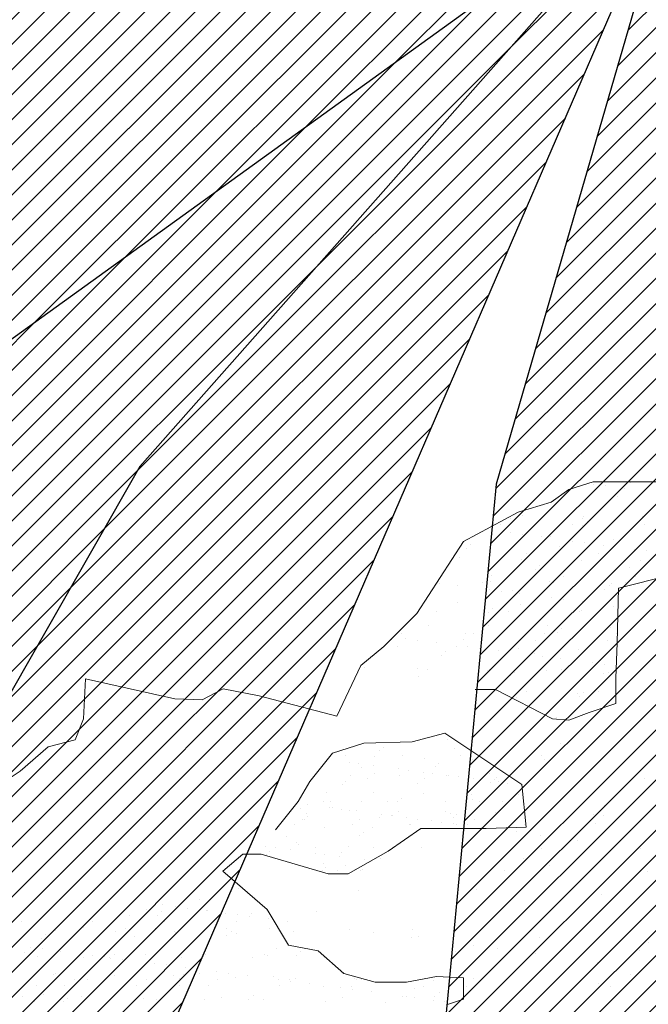
# Model space of a CAD drawing. Units: inches. Extents: x 1986 to 21484, y -1816 to 2016.
# Tile 16 of 85: x 2166.564 to 2172.013, y 1873.899 to 1882.437. Entities that reach past the tile are written whole.
import ezdxf

# ---------------------------------------------------------------- set-up
doc = ezdxf.new("R2010")
doc.units = ezdxf.units.IN
doc.layers.add('L-PLNT', color=84, linetype='Continuous', lineweight=13)
doc.layers.add('vfolhas', color=114, linetype='Continuous', lineweight=5)
doc.layers.add('vfolha', color=72, linetype='Continuous')
doc.layers.add('vfolha2', color=110, linetype='Continuous')
pattern_1 = [(45, (-2446.5133113, 50.986076), (-0.004419417382, 0.004419417382), [])]

# ---------------------------------------------------------------- blocks, each defined once
blk = doc.blocks.new('arbusto_PB_verde_grande')
at = {"layer": 'vfolha2'}
h = blk.add_hatch(dxfattribs=at)
h.set_pattern_fill('ANSI31', color=256, scale=0.05, style=0)
h.set_pattern_definition(pattern_1)
h.paths.add_polyline_path([(0.02944, 0.35651), (0.00028, 0.09048), (0.02625, -0.03934), (0.047, 0.06233), (0.06189, 0.09731), (0.09372, 0.26573), (0.09955, 0.43473), (0.08789, 0.61313), (0.0645, 0.72266), (0.04988, 0.6851), (0.0236, 0.51294)])
h.paths.add_polyline_path([(0.30106, 0.43789), (0.14225, 0.24871), (0.26685, 0.30022)])
h.paths.add_polyline_path([(0.37995, 0.22817), (0.23697, 0.15193), (0.18428, 0.09364), (0.11122, 0.04358), (0.02625, -0.03934), (0.28061, 0.04667), (0.36829, 0.07798), (0.46756, 0.11239), (0.61068, 0.19376), (0.71585, 0.27823), (0.55813, 0.25948)])
h.paths.add_polyline_path([(0.56101, -0.29441), (0.72752, -0.32573), (0.59024, -0.2412), (0.42962, -0.15982), (0.02625, -0.03934), (0.14922, -0.14107), (0.18838, -0.16604), (0.41501, -0.24435)])
h.paths.add_polyline_path([(-0.27429, -0.44776), (-0.30352, -0.72628), (-0.23923, -0.64175), (-0.15457, -0.45716), (0.02625, -0.03934), (-0.16328, -0.25376)])
h.paths.add_polyline_path([(-0.51963, -0.24744), (-0.67736, -0.32573), (-0.59558, -0.35072), (-0.40574, -0.32882), (-0.21007, -0.20995), (0.02625, -0.03934), (-0.14874, -0.06595), (-0.31518, -0.09101), (-0.41452, -0.15048)])
h.paths.add_polyline_path([(-0.52546, 0.25007), (-0.70947, 0.24698), (-0.51963, 0.1093), (-0.32979, 0.02167), (-0.07567, -0.0128), (-0.04234, -0.02148), (-0.35024, 0.1312)])
at = {"layer": 'vfolhas'}
h = blk.add_hatch(dxfattribs=at)
h.set_pattern_fill('ANSI31', color=256, scale=0.05, style=0)
h.set_pattern_definition(pattern_1)
h.paths.add_polyline_path([(-0.07279, 0.50669), (-0.18085, 0.65063), (-0.2334, 0.67253), (-0.20712, 0.53176), (-0.10785, 0.25007), (0.02625, -0.03934), (0.00028, 0.09048), (0.00816, 0.16241), (-0.04939, 0.29079)])
h.paths.add_polyline_path([(0.09902, 0.41929), (0.09372, 0.26573), (0.07906, 0.18814), (0.15506, 0.36901), (0.26606, 0.5505), (0.28356, 0.63504), (0.2485, 0.68819), (0.25145, 0.63504), (0.20178, 0.54426)])
h.paths.add_polyline_path([(0.12295, 0.24073), (0.047, 0.06233), (0.02625, -0.03934), (0.11122, 0.04358), (0.18428, 0.09364), (0.27478, 0.19376), (0.3215, 0.25323), (0.44129, 0.38467), (0.47634, 0.57866), (0.41789, 0.45347), (0.28939, 0.30954)])
h.paths.add_polyline_path([(0.58145, -0.03779), (0.70707, 0.01536), (0.78591, 0.04667), (0.74796, 0.06549), (0.62818, 0.08423), (0.52595, 0.09048), (0.39745, 0.04358), (0.02625, -0.03934), (0.25728, -0.03154), (0.43834, -0.0347)])
h.paths.add_polyline_path([(0.52022, -0.03647), (0.43834, -0.0347), (0.25728, -0.03154), (0.02625, -0.03934), (0.17964, -0.08515), (0.53768, -0.13167), (0.69541, -0.15357), (0.78591, -0.07852), (0.70413, -0.10042)])
h.paths.add_polyline_path([(0.27189, -0.21929), (0.14922, -0.14107), (0.02625, -0.03934), (0.15794, -0.31007), (0.29522, -0.42585), (0.41789, -0.49157), (0.56396, -0.56669), (0.5114, -0.48532), (0.39456, -0.34139)])
h.paths.add_polyline_path([(-0.05818, -0.47591), (-0.02312, -0.61984), (0.047, -0.80134), (0.08494, -0.59794), (0.07911, -0.4071), (0.03527, -0.25376), (0.02625, -0.03934), (-0.03773, -0.26001)])
h.paths.add_polyline_path([(-0.24218, 0.14054), (-0.11073, 0.06858), (0.02625, -0.03934), (-0.04235, 0.10871), (-0.21007, 0.23757), (-0.36485, 0.33145), (-0.47874, 0.40341), (-0.54303, 0.46288), (-0.49041, 0.33145), (-0.39408, 0.22192)])
h = blk.add_hatch(dxfattribs=at)
h.set_pattern_fill('ANSI31', color=256, scale=0.05, style=0)
h.set_pattern_definition(pattern_1)
h.paths.add_polyline_path([(-0.57219, 0.06233), (-0.7153, 0.10298), (-0.67736, 0.08107), (-0.62769, 0.01536), (-0.56347, -0.04095), (-0.26461, -0.0834), (-0.14874, -0.06595), (-0.10151, -0.05877), (-0.20418, -0.0472), (-0.40279, -0.00339)])
h.paths.add_polyline_path([(-0.56347, -0.04095), (-0.58279, -0.02401), (-0.72992, -0.09726), (-0.4334, -0.1679), (-0.41452, -0.15048), (-0.31518, -0.09101), (-0.26461, -0.0834)])
h.paths.add_polyline_path([(-0.2769, -0.47267), (-0.27429, -0.44776), (-0.16328, -0.25376), (0.02625, -0.03934), (-0.21007, -0.20995), (-0.2672, -0.24466), (-0.36485, -0.35697), (-0.42907, -0.46341), (-0.47586, -0.60425), (-0.37946, -0.57603)])
at = {"layer": 'vfolha'}
for p, q in [((0.02625, -0.03934), (-0.03773, -0.26001)), ((-0.03773, -0.26001), (-0.05818, -0.47591))]:
    blk.add_line(p, q, dxfattribs=at)
at = {"layer": 'vfolha2'}
for p, q in [((-0.21007, -0.20995), (0.02625, -0.03934)), ((0.02625, -0.03934), (-0.16328, -0.25376)), ((-0.15457, -0.45716), (0.02625, -0.03934)), ((-0.16328, -0.25376), (-0.27429, -0.44776))]:
    blk.add_line(p, q, dxfattribs=at)
blk = doc.blocks.new('PLANT-SHRUB')
for p, q in [((2171.3247, 1878.3633), (2171.5336, 1878.4292)), ((2171.5336, 1878.4292), (2172.7926, 1878.4292)), ((2171.5405, 1878.409), (2171.5405, 1878.409)), ((2171.6445, 1878.3953), (2171.6445, 1878.3953)), ((2171.807, 1878.3739), (2171.807, 1878.3739)), ((2171.8549, 1878.4232), (2171.8549, 1878.4232)), ((2171.1708, 1878.2535), (2171.3247, 1878.3633)), ((2171.7198, 1878.3176), (2171.7198, 1878.3176)), ((2171.7435, 1878.3055), (2171.7435, 1878.3055)), ((2170.8849, 1878.1656), (2171.1708, 1878.2535)), ((2171.656, 1878.241), (2171.656, 1878.241)), ((2170.4122, 1877.9129), (2170.8849, 1878.1656)), ((2170.8178, 1878.1134), (2170.8178, 1878.1134)), ((2170.9265, 1878.1369), (2170.9265, 1878.1369)), ((2171.4401, 1878.1123), (2171.4401, 1878.1123)), ((2171.4496, 1878.1303), (2171.4496, 1878.1303)), ((2171.9608, 1878.1327), (2171.9608, 1878.1327)), ((2170.7335, 1878.0597), (2170.7335, 1878.0597)), ((2171.3558, 1878.0586), (2171.3558, 1878.0586)), ((2171.4453, 1878.0479), (2171.4453, 1878.0479)), ((2171.4822, 1878.0816), (2171.4822, 1878.0816)), ((2171.9781, 1878.0575), (2171.9781, 1878.0575)), ((2170.6563, 1877.9496), (2170.6563, 1877.9496)), ((2170.8183, 1877.9867), (2170.8183, 1877.9867)), ((2170.9224, 1877.973), (2170.9224, 1877.973)), ((2171.0848, 1877.9516), (2171.0848, 1877.9516)), ((2171.1675, 1877.952), (2171.1675, 1877.952)), ((2170.0053, 1877.2867), (2170.4122, 1877.9129)), ((2170.4718, 1877.8817), (2170.4718, 1877.8817)), ((2171.2464, 1877.8656), (2171.2464, 1877.8656)), ((2171.3563, 1877.9159), (2171.3563, 1877.9159)), ((2171.4603, 1877.9022), (2171.4603, 1877.9022)), ((2171.6227, 1877.8808), (2171.6227, 1877.8808)), ((2171.7072, 1877.9326), (2171.7072, 1877.9326)), ((2170.3742, 1877.7713), (2170.3742, 1877.7713)), ((2170.435, 1877.848), (2170.435, 1877.848)), ((2170.9598, 1877.8063), (2170.9598, 1877.8063)), ((2171.5821, 1877.8051), (2171.5821, 1877.8051)), ((2171.8942, 1877.845), (2171.8942, 1877.845)), ((2171.9982, 1877.8313), (2171.9982, 1877.8313)), ((2170.9139, 1877.7519), (2170.9139, 1877.7519)), ((2171.0726, 1877.7063), (2171.0726, 1877.7063)), ((2171.437, 1877.7452), (2171.437, 1877.7452)), ((2171.8472, 1877.6902), (2171.8472, 1877.6902)), ((2171.9482, 1877.7477), (2171.9482, 1877.7477)), ((2170.6564, 1877.613), (2170.6564, 1877.613)), ((2171.0357, 1877.6726), (2171.0357, 1877.6726)), ((2171.2787, 1877.6119), (2171.2787, 1877.6119)), ((2172.3518, 1877.6562), (2171.7549, 1877.5082)), ((2171.901, 1877.6107), (2171.901, 1877.6107)), ((2170.2002, 1877.5506), (2170.2002, 1877.5506)), ((2170.3627, 1877.5293), (2170.3627, 1877.5293)), ((2170.5721, 1877.5593), (2170.5721, 1877.5593)), ((2170.6437, 1877.5645), (2170.6437, 1877.5645)), ((2171.1549, 1877.567), (2171.1549, 1877.567)), ((2171.1944, 1877.5582), (2171.1944, 1877.5582)), ((2171.6733, 1877.5309), (2171.6733, 1877.5309)), ((2171.6946, 1877.5475), (2171.6946, 1877.5475)), ((2171.8168, 1877.5571), (2171.8168, 1877.5571)), ((2170.6341, 1877.4935), (2170.6341, 1877.4935)), ((2170.7381, 1877.4798), (2170.7381, 1877.4798)), ((2170.8368, 1877.4903), (2170.8368, 1877.4903)), ((2170.9006, 1877.4584), (2170.9006, 1877.4584)), ((2171.6365, 1877.4972), (2171.6365, 1877.4972)), ((2171.7549, 1877.5082), (2171.7425, 1877.034)), ((2170.3616, 1877.3863), (2170.3616, 1877.3863)), ((2170.9013, 1877.3668), (2170.9013, 1877.3668)), ((2171.172, 1877.4227), (2171.172, 1877.4227)), ((2171.276, 1877.409), (2171.276, 1877.409)), ((2171.4244, 1877.3602), (2171.4244, 1877.3602)), ((2171.4385, 1877.3876), (2171.4385, 1877.3876)), ((2171.7099, 1877.3519), (2171.7099, 1877.3519)), ((2169.7195, 1877.001), (2170.0053, 1877.2867)), ((2170.1761, 1877.307), (2170.1761, 1877.307)), ((2170.6262, 1877.2973), (2170.6262, 1877.2973)), ((2170.663, 1877.331), (2170.663, 1877.331)), ((2170.7984, 1877.3059), (2170.7984, 1877.3059)), ((2171.4207, 1877.3047), (2171.4207, 1877.3047)), ((2171.4376, 1877.3149), (2171.4376, 1877.3149)), ((2170.108, 1877.1862), (2170.108, 1877.1862)), ((2170.6311, 1877.1795), (2170.6311, 1877.1795)), ((2171.1423, 1877.1819), (2171.1423, 1877.1819)), ((2169.8727, 1877.1137), (2169.8727, 1877.1137)), ((2170.4273, 1877.115), (2170.4273, 1877.115)), ((2170.495, 1877.1126), (2170.495, 1877.1126)), ((2171.1173, 1877.1115), (2171.1173, 1877.1115)), ((2171.2269, 1877.1219), (2171.2269, 1877.1219)), ((2171.2637, 1877.1556), (2171.2637, 1877.1556)), ((2171.682, 1877.1625), (2171.682, 1877.1625)), ((2171.7396, 1877.1103), (2171.7396, 1877.1103)), ((2169.5216, 1876.8362), (2169.7195, 1877.001)), ((2169.7884, 1877.06), (2169.7884, 1877.06)), ((2169.8378, 1876.9988), (2169.8378, 1876.9988)), ((2169.9119, 1877.0712), (2169.9119, 1877.0712)), ((2170.016, 1877.0575), (2170.016, 1877.0575)), ((2170.1784, 1877.0361), (2170.1784, 1877.0361)), ((2170.349, 1877.0012), (2170.349, 1877.0012)), ((2170.4107, 1877.0589), (2170.4107, 1877.0589)), ((2170.4498, 1877.0004), (2170.4498, 1877.0004)), ((2171.033, 1877.0578), (2171.033, 1877.0578)), ((2171.6554, 1877.0566), (2171.6554, 1877.0566)), ((2171.7425, 1877.034), (2171.7315, 1876.7264)), ((2170.2166, 1876.9219), (2170.2166, 1876.9219)), ((2170.2534, 1876.9557), (2170.2534, 1876.9557)), ((2170.5539, 1876.9867), (2170.5539, 1876.9867)), ((2170.7163, 1876.9653), (2170.7163, 1876.9653)), ((2170.8887, 1876.9818), (2170.8887, 1876.9818)), ((2170.9878, 1876.9296), (2170.9878, 1876.9296)), ((2171.028, 1876.9396), (2171.028, 1876.9396)), ((2171.0918, 1876.9159), (2171.0918, 1876.9159)), ((2171.4118, 1876.9751), (2171.4118, 1876.9751)), ((2169.3127, 1876.3968), (2169.5216, 1876.8362)), ((2171.2542, 1876.8945), (2171.2542, 1876.8945)), ((2171.5257, 1876.8587), (2171.5257, 1876.8587)), ((2171.6297, 1876.845), (2171.6297, 1876.845)), ((2169.5557, 1876.8206), (2169.5557, 1876.8206)), ((2170.0147, 1876.8066), (2170.0147, 1876.8066)), ((2170.0954, 1876.8011), (2170.0954, 1876.8011)), ((2170.6185, 1876.7944), (2170.6185, 1876.7944)), ((2170.637, 1876.8055), (2170.637, 1876.8055)), ((2170.8173, 1876.7465), (2170.8173, 1876.7465)), ((2170.8541, 1876.7803), (2170.8541, 1876.7803)), ((2171.1297, 1876.7969), (2171.1297, 1876.7969)), ((2171.2593, 1876.8043), (2171.2593, 1876.8043)), ((2171.6287, 1876.7642), (2171.6287, 1876.7642)), ((2171.6694, 1876.7774), (2171.6694, 1876.7774)), ((2167.1158, 1876.3736), (2167.1332, 1876.7213)), ((2167.1332, 1876.7213), (2167.9098, 1876.5474)), ((2170.0177, 1876.7397), (2170.0177, 1876.7397)), ((2171.7315, 1876.7264), (2171.7315, 1876.5067)), ((2168.1447, 1876.5387), (2168.3274, 1876.6343)), ((2168.3274, 1876.6343), (2168.6406, 1876.5735)), ((2168.6406, 1876.5735), (2169.3127, 1876.3968)), ((2170.687, 1876.6275), (2170.5111, 1876.6275)), ((2171.1818, 1876.3748), (2170.687, 1876.6275)), ((2170.8761, 1876.5968), (2170.8761, 1876.5968)), ((2170.9559, 1876.6111), (2170.9559, 1876.6111)), ((2171.3992, 1876.5901), (2171.3992, 1876.5901)), ((2171.418, 1876.5712), (2171.418, 1876.5712)), ((2171.4549, 1876.6049), (2171.4549, 1876.6049)), ((2171.5782, 1876.6099), (2171.5782, 1876.6099)), ((2167.9098, 1876.5474), (2168.1447, 1876.5387)), ((2170.8717, 1876.5574), (2170.8717, 1876.5574)), ((2171.494, 1876.5562), (2171.494, 1876.5562)), ((2171.7315, 1876.5067), (2171.5006, 1876.4298)), ((2171.1171, 1876.4118), (2171.1171, 1876.4118)), ((2171.5006, 1876.4298), (2171.3247, 1876.3638)), ((2167.0462, 1876.191), (2167.1158, 1876.3736)), ((2169.3127, 1876.3968), (2169.3127, 1876.3968)), ((2171.3247, 1876.3638), (2171.1818, 1876.3748)), ((2171.2191, 1876.3889), (2171.2191, 1876.3889)), ((2170.2504, 1876.25), (2169.9665, 1876.176)), ((2170.9168, 1875.8061), (2170.2504, 1876.25)), ((2166.8113, 1876.1302), (2167.0462, 1876.191)), ((2169.5469, 1876.1637), (2169.2754, 1876.0773)), ((2169.9665, 1876.176), (2169.5469, 1876.1637)), ((2169.5469, 1876.1637), (2169.5469, 1876.1637)), ((2170.2731, 1876.1911), (2170.2731, 1876.1911)), ((2171.2553, 1876.1632), (2171.2553, 1876.1632)), ((2166.5677, 1875.9215), (2166.8113, 1876.1302)), ((2169.2754, 1876.0773), (2169.0779, 1875.8307)), ((2169.6868, 1876.1011), (2169.6868, 1876.1011)), ((2169.7163, 1876.1281), (2169.7163, 1876.1281)), ((2170.336, 1876.1153), (2170.336, 1876.1153)), ((2169.387, 1876.0573), (2169.387, 1876.0573)), ((2169.4198, 1875.9977), (2169.4198, 1875.9977)), ((2169.503, 1875.9867), (2169.503, 1875.9867)), ((2169.6384, 1876.0466), (2169.6384, 1876.0466)), ((2169.8848, 1876.0564), (2169.8848, 1876.0564)), ((2170.0702, 1876.031), (2170.0702, 1876.031)), ((2170.1969, 1875.9878), (2170.1969, 1875.9878)), ((2170.3827, 1876.0555), (2170.3827, 1876.0555)), ((2170.4887, 1876.0257), (2170.4887, 1876.0257)), ((2171.0868, 1876.0558), (2171.0868, 1876.0558)), ((2171.1164, 1876.0177), (2171.1164, 1876.0177)), ((2166.3589, 1875.7824), (2166.5677, 1875.9215)), ((2169.5277, 1875.9553), (2169.5277, 1875.9553)), ((2169.633, 1875.9696), (2169.633, 1875.9696)), ((2169.6421, 1875.9018), (2169.6421, 1875.9018)), ((2169.8501, 1875.941), (2169.8501, 1875.941)), ((2169.9334, 1875.9301), (2169.9334, 1875.9301)), ((2170.0633, 1875.913), (2170.0633, 1875.913)), ((2170.14, 1875.9009), (2170.14, 1875.9009)), ((2170.1674, 1875.9608), (2170.1674, 1875.9608)), ((2170.6378, 1875.9), (2170.6378, 1875.9)), ((2169.0779, 1875.8307), (2168.9792, 1875.6581)), ((2169.3886, 1875.8279), (2169.3886, 1875.8279)), ((2169.4356, 1875.8865), (2169.4356, 1875.8865)), ((2169.5747, 1875.8588), (2169.5747, 1875.8588)), ((2169.8541, 1875.8811), (2169.8541, 1875.8811)), ((2170.0083, 1875.815), (2170.0083, 1875.815)), ((2170.0725, 1875.8579), (2170.0725, 1875.8579)), ((2170.263, 1875.8831), (2170.263, 1875.8831)), ((2170.2805, 1875.8844), (2170.2805, 1875.8844)), ((2170.3637, 1875.8734), (2170.3637, 1875.8734)), ((2170.4937, 1875.8563), (2170.4937, 1875.8563)), ((2170.5704, 1875.857), (2170.5704, 1875.857)), ((2170.648, 1875.8205), (2170.648, 1875.8205)), ((2170.6775, 1875.8475), (2170.6775, 1875.8475)), ((2170.6948, 1875.8675), (2170.6948, 1875.8675)), ((2170.7108, 1875.8277), (2170.7108, 1875.8277)), ((2170.794, 1875.8168), (2170.794, 1875.8168)), ((2170.9538, 1875.4361), (2170.9168, 1875.8061)), ((2171.9759, 1875.8559), (2171.9759, 1875.8559)), ((2169.2194, 1875.7366), (2169.2194, 1875.7366)), ((2169.3592, 1875.8009), (2169.3592, 1875.8009)), ((2169.6284, 1875.7385), (2169.6284, 1875.7385)), ((2170.0602, 1875.723), (2170.0602, 1875.723)), ((2170.4786, 1875.7176), (2170.4786, 1875.7176)), ((2170.8876, 1875.7196), (2170.8876, 1875.7196)), ((2168.9792, 1875.6581), (2168.7818, 1875.4114)), ((2169.0553, 1875.6318), (2169.0553, 1875.6318)), ((2169.2001, 1875.6551), (2169.2001, 1875.6551)), ((2169.2578, 1875.657), (2169.2578, 1875.657)), ((2169.5298, 1875.6563), (2169.5298, 1875.6563)), ((2169.7557, 1875.6561), (2169.7557, 1875.6561)), ((2169.8398, 1875.6606), (2169.8398, 1875.6606)), ((2169.8692, 1875.6876), (2169.8692, 1875.6876)), ((2170.2535, 1875.6552), (2170.2535, 1875.6552)), ((2170.4889, 1875.6747), (2170.4889, 1875.6747)), ((2170.5522, 1875.6612), (2170.5522, 1875.6612)), ((2170.7514, 1875.6543), (2170.7514, 1875.6543)), ((2168.9937, 1875.594), (2168.9937, 1875.594)), ((2169.05, 1875.5534), (2169.05, 1875.5534)), ((2169.2502, 1875.6061), (2169.2502, 1875.6061)), ((2169.2724, 1875.6032), (2169.2724, 1875.6032)), ((2169.3556, 1875.5922), (2169.3556, 1875.5922)), ((2169.4255, 1875.5784), (2169.4255, 1875.5784)), ((2169.4856, 1875.5751), (2169.4856, 1875.5751)), ((2169.7027, 1875.5465), (2169.7027, 1875.5465)), ((2169.844, 1875.5731), (2169.844, 1875.5731)), ((2170.2529, 1875.575), (2170.2529, 1875.575)), ((2170.2946, 1875.5512), (2170.2946, 1875.5512)), ((2170.3498, 1875.5473), (2170.3498, 1875.5473)), ((2170.6847, 1875.5595), (2170.6847, 1875.5595)), ((2171.5393, 1875.5489), (2171.5393, 1875.5489)), ((2171.6317, 1875.6223), (2171.6317, 1875.6223)), ((2169.0151, 1875.5024), (2169.0151, 1875.5024)), ((2169.0315, 1875.5006), (2169.0315, 1875.5006)), ((2169.061, 1875.5276), (2169.061, 1875.5276)), ((2169.513, 1875.5015), (2169.513, 1875.5015)), ((2169.6806, 1875.5148), (2169.6806, 1875.5148)), ((2169.786, 1875.5356), (2169.786, 1875.5356)), ((2169.7931, 1875.5346), (2169.7931, 1875.5346)), ((2169.9159, 1875.5185), (2169.9159, 1875.5185)), ((2170.0108, 1875.5005), (2170.0108, 1875.5005)), ((2170.1331, 1875.4899), (2170.1331, 1875.4899)), ((2170.2163, 1875.4789), (2170.2163, 1875.4789)), ((2170.3203, 1875.5203), (2170.3203, 1875.5203)), ((2170.326, 1875.4645), (2170.326, 1875.4645)), ((2170.3463, 1875.4618), (2170.3463, 1875.4618)), ((2170.5087, 1875.4996), (2170.5087, 1875.4996)), ((2171.5545, 1875.4697), (2171.5545, 1875.4697)), ((2171.6282, 1875.5372), (2171.6282, 1875.5372)), ((2168.9477, 1875.4594), (2168.9477, 1875.4594)), ((2169.2093, 1875.4285), (2169.2093, 1875.4285)), ((2169.4456, 1875.4585), (2169.4456, 1875.4585)), ((2169.5416, 1875.3873), (2169.5416, 1875.3873)), ((2169.6183, 1875.4305), (2169.6183, 1875.4305)), ((2169.7567, 1875.2265), (2170.0406, 1875.4238)), ((2169.9434, 1875.4576), (2169.9434, 1875.4576)), ((2169.9553, 1875.456), (2169.9553, 1875.456)), ((2170.0406, 1875.4238), (2170.6083, 1875.4238)), ((2170.4413, 1875.4567), (2170.4413, 1875.4567)), ((2170.5634, 1875.4332), (2170.5634, 1875.4332)), ((2170.6083, 1875.4238), (2170.9538, 1875.4361)), ((2170.8689, 1875.393), (2170.8689, 1875.393)), ((2170.9391, 1875.4558), (2170.9391, 1875.4558)), ((2168.8724, 1875.3548), (2168.8724, 1875.3548)), ((2168.9656, 1875.2998), (2168.9656, 1875.2998)), ((2169.5121, 1875.3603), (2169.5121, 1875.3603)), ((2171.0769, 1875.3656), (2171.0769, 1875.3656)), ((2171.4019, 1875.3228), (2171.4019, 1875.3228)), ((2168.6947, 1875.2653), (2168.6947, 1875.2653)), ((2168.7333, 1875.2274), (2168.7333, 1875.2274)), ((2168.7779, 1875.2544), (2168.7779, 1875.2544)), ((2168.9079, 1875.2372), (2168.9079, 1875.2372)), ((2168.9837, 1875.2859), (2168.9837, 1875.2859)), ((2169.125, 1875.2087), (2169.125, 1875.2087)), ((2169.1287, 1875.2566), (2169.1287, 1875.2566)), ((2169.353, 1875.2145), (2169.353, 1875.2145)), ((2169.4112, 1875.0292), (2169.7567, 1875.2265)), ((2169.4154, 1875.2704), (2169.4154, 1875.2704)), ((2169.6266, 1875.2557), (2169.6266, 1875.2557)), ((2170.0451, 1875.2609), (2170.0451, 1875.2609)), ((2171.0912, 1875.2476), (2171.0912, 1875.2476)), ((2171.9447, 1875.2514), (2171.9447, 1875.2514)), ((2168.3251, 1875.0538), (2168.4979, 1875.2018)), ((2168.4979, 1875.2018), (2168.6583, 1875.2018)), ((2168.6583, 1875.2018), (2169.2384, 1875.0292)), ((2168.7038, 1875.2004), (2168.7038, 1875.2004)), ((2169.1993, 1875.1205), (2169.1993, 1875.1205)), ((2169.2082, 1875.1977), (2169.2082, 1875.1977)), ((2169.3382, 1875.1806), (2169.3382, 1875.1806)), ((2169.5553, 1875.152), (2169.5553, 1875.152)), ((2169.6075, 1875.1374), (2169.6075, 1875.1374)), ((2169.6879, 1875.1646), (2169.6879, 1875.1646)), ((2170.9325, 1875.1624), (2170.9325, 1875.1624)), ((2168.3251, 1875.0538), (2168.3251, 1875.0538)), ((2168.7077, 1874.7209), (2168.3251, 1875.0538)), ((2169.1844, 1875.0601), (2169.1844, 1875.0601)), ((2169.2139, 1875.0871), (2169.2139, 1875.0871)), ((2169.3165, 1875.0582), (2169.3165, 1875.0582)), ((2169.3839, 1875.1011), (2169.3839, 1875.1011)), ((2169.5194, 1875.0573), (2169.5194, 1875.0573)), ((2169.5339, 1875.0699), (2169.5339, 1875.0699)), ((2170.764, 1875.055), (2170.764, 1875.055)), ((2171.1567, 1875.1052), (2171.1567, 1875.1052)), ((2172.0086, 1875.0527), (2172.0086, 1875.0527)), ((2169.2384, 1875.0292), (2169.4112, 1875.0292)), ((2168.4584, 1874.8995), (2168.4584, 1874.8995)), ((2168.4584, 1874.8995), (2168.4584, 1874.8995)), ((2169.5046, 1874.8862), (2169.5046, 1874.8862)), ((2170.527, 1874.8911), (2170.527, 1874.8911)), ((2168.1245, 1874.8072), (2168.1245, 1874.8072)), ((2170.809, 1874.7866), (2170.809, 1874.7866)), ((2171.6065, 1874.8522), (2171.6065, 1874.8522)), ((2167.6651, 1874.7188), (2167.6651, 1874.7188)), ((2167.7959, 1874.7038), (2167.7959, 1874.7038)), ((2167.8059, 1874.7614), (2167.8059, 1874.7614)), ((2167.9149, 1874.7471), (2167.9149, 1874.7471)), ((2168.0189, 1874.7334), (2168.0189, 1874.7334)), ((2168.1814, 1874.712), (2168.1814, 1874.712)), ((2168.1882, 1874.7122), (2168.1882, 1874.7122)), ((2168.6994, 1874.7146), (2168.6994, 1874.7146)), ((2168.8928, 1874.4126), (2168.7077, 1874.7209)), ((2169.1361, 1874.7054), (2169.1361, 1874.7054)), ((2170.7353, 1874.7191), (2170.7353, 1874.7191)), ((2166.5765, 1874.6162), (2166.5765, 1874.6162)), ((2167.1988, 1874.6151), (2167.1988, 1874.6151)), ((2167.5132, 1874.67), (2167.5132, 1874.67)), ((2167.759, 1874.67), (2167.759, 1874.67)), ((2167.8211, 1874.6139), (2167.8211, 1874.6139)), ((2168.3488, 1874.69), (2168.3488, 1874.69)), ((2168.4434, 1874.6128), (2168.4434, 1874.6128)), ((2168.4528, 1874.6763), (2168.4528, 1874.6763)), ((2168.5568, 1874.6626), (2168.5568, 1874.6626)), ((2168.5568, 1874.6626), (2168.5568, 1874.6626)), ((2168.5705, 1874.6877), (2168.5705, 1874.6877)), ((2168.7193, 1874.6412), (2168.7193, 1874.6412)), ((2168.8817, 1874.6198), (2168.8817, 1874.6198)), ((2166.8718, 1874.5382), (2166.8718, 1874.5382)), ((2166.8718, 1874.5382), (2166.8718, 1874.5382)), ((2167.1145, 1874.5614), (2167.1145, 1874.5614)), ((2167.3949, 1874.5315), (2167.3949, 1874.5315)), ((2167.4826, 1874.5549), (2167.4826, 1874.5549)), ((2167.7368, 1874.5603), (2167.7368, 1874.5603)), ((2167.9061, 1874.5339), (2167.9061, 1874.5339)), ((2167.918, 1874.5248), (2167.918, 1874.5248)), ((2168.3591, 1874.5591), (2168.3591, 1874.5591)), ((2168.3966, 1874.5284), (2168.3966, 1874.5284)), ((2168.7272, 1874.5526), (2168.7272, 1874.5526)), ((2168.9404, 1874.5297), (2168.9404, 1874.5297)), ((2169.4246, 1874.5483), (2169.4246, 1874.5483)), ((2169.9719, 1874.5504), (2169.9719, 1874.5504)), ((2171.2165, 1874.5481), (2171.2165, 1874.5481)), ((2166.7487, 1874.4701), (2166.7487, 1874.4701)), ((2166.7855, 1874.5038), (2166.7855, 1874.5038)), ((2167.5601, 1874.4878), (2167.5601, 1874.4878)), ((2168.3598, 1874.4946), (2168.3598, 1874.4946)), ((2168.4459, 1874.5145), (2168.4459, 1874.5145)), ((2169.6326, 1874.5209), (2169.6326, 1874.5209)), ((2169.9576, 1874.4782), (2169.9576, 1874.4782)), ((2170.0199, 1874.4908), (2170.0199, 1874.4908)), ((2171.0661, 1874.4775), (2171.0661, 1874.4775)), ((2166.6016, 1874.3508), (2166.6016, 1874.3508)), ((2166.6548, 1874.3956), (2166.6548, 1874.3956)), ((2166.7588, 1874.3819), (2166.7588, 1874.3819)), ((2166.9213, 1874.3605), (2166.9213, 1874.3605)), ((2167.1128, 1874.3532), (2167.1128, 1874.3532)), ((2168.7884, 1874.3867), (2168.7884, 1874.3867)), ((2169.152, 1874.3632), (2168.8928, 1874.4126)), ((2168.9973, 1874.353), (2168.9973, 1874.353)), ((2169.3741, 1874.1659), (2169.152, 1874.3632)), ((2170.3375, 1874.3546), (2170.3375, 1874.3546)), ((2170.5004, 1874.4067), (2170.5004, 1874.4067)), ((2170.7085, 1874.3793), (2170.7085, 1874.3793)), ((2171.9368, 1874.3683), (2171.9368, 1874.3683)), ((2172.0105, 1874.4358), (2172.0105, 1874.4358)), ((2166.7184, 1874.3091), (2166.7184, 1874.3091)), ((2167.1154, 1874.3055), (2167.1154, 1874.3055)), ((2167.1927, 1874.3248), (2167.1927, 1874.3248)), ((2167.2967, 1874.3111), (2167.2967, 1874.3111)), ((2167.3407, 1874.3079), (2167.3407, 1874.3079)), ((2167.3494, 1874.2947), (2167.3494, 1874.2947)), ((2167.3863, 1874.3284), (2167.3863, 1874.3284)), ((2167.4592, 1874.2897), (2167.4592, 1874.2897)), ((2167.6526, 1874.3338), (2167.6526, 1874.3338)), ((2167.9631, 1874.3068), (2167.9631, 1874.3068)), ((2168.1609, 1874.3124), (2168.1609, 1874.3124)), ((2168.1756, 1874.3271), (2168.1756, 1874.3271)), ((2168.5854, 1874.3057), (2168.5854, 1874.3057)), ((2168.6868, 1874.3296), (2168.6868, 1874.3296)), ((2168.7147, 1874.3192), (2168.7147, 1874.3192)), ((2168.9605, 1874.3192), (2168.9605, 1874.3192)), ((2169.2077, 1874.3045), (2169.2077, 1874.3045)), ((2171.0334, 1874.3365), (2171.0334, 1874.3365)), ((2167.7306, 1874.2539), (2167.7306, 1874.2539)), ((2167.8346, 1874.2402), (2167.8346, 1874.2402)), ((2167.9971, 1874.2189), (2167.9971, 1874.2189)), ((2168.2685, 1874.1831), (2168.2685, 1874.1831)), ((2171.5762, 1874.2651), (2171.5762, 1874.2651)), ((2171.7843, 1874.2377), (2171.7843, 1874.2377)), ((2166.8592, 1874.1531), (2166.8592, 1874.1531)), ((2166.8758, 1874.1683), (2166.8758, 1874.1683)), ((2167.0374, 1874.1147), (2167.0374, 1874.1147)), ((2167.1505, 1874.1124), (2167.1505, 1874.1124)), ((2167.3538, 1874.1683), (2167.3538, 1874.1683)), ((2167.3823, 1874.1464), (2167.3823, 1874.1464)), ((2167.6597, 1874.1135), (2167.6597, 1874.1135)), ((2167.8935, 1874.1489), (2167.8935, 1874.1489)), ((2167.9502, 1874.1193), (2167.9502, 1874.1193)), ((2167.987, 1874.1531), (2167.987, 1874.1531)), ((2168.1205, 1874.1661), (2168.1205, 1874.1661)), ((2168.282, 1874.1124), (2168.282, 1874.1124)), ((2168.3726, 1874.1694), (2168.3726, 1874.1694)), ((2168.4333, 1874.1294), (2168.4333, 1874.1294)), ((2168.4333, 1874.1294), (2168.4333, 1874.1294)), ((2168.535, 1874.148), (2168.535, 1874.148)), ((2168.7616, 1874.137), (2168.7616, 1874.137)), ((2168.8065, 1874.1123), (2168.8065, 1874.1123)), ((2168.9043, 1874.1113), (2168.9043, 1874.1113)), ((2168.9105, 1874.0986), (2168.9105, 1874.0986)), ((2168.9564, 1874.1228), (2168.9564, 1874.1228)), ((2169.3651, 1874.1638), (2169.3651, 1874.1638)), ((2169.6456, 1874.0919), (2169.3741, 1874.1659)), ((2169.4676, 1874.1252), (2169.4676, 1874.1252)), ((2169.4794, 1874.1161), (2169.4794, 1874.1161)), ((2169.5266, 1874.1101), (2169.5266, 1874.1101)), ((2170.1763, 1874.1413), (2169.9172, 1874.0919)), ((2170.0073, 1874.1058), (2170.0073, 1874.1058)), ((2170.149, 1874.109), (2170.149, 1874.109)), ((2170.4108, 1874.1289), (2170.1763, 1874.1413)), ((2170.4108, 1874.1289), (2170.4108, 1874.1289)), ((2170.4108, 1873.944), (2170.4108, 1874.1289)), ((2170.5018, 1874.121), (2170.5018, 1874.121)), ((2170.6097, 1874.1616), (2170.6097, 1874.1616)), ((2171.8544, 1874.1593), (2171.8544, 1874.1593)), ((2166.7073, 1874.061), (2166.7073, 1874.061)), ((2166.9531, 1874.061), (2166.9531, 1874.061)), ((2167.5754, 1874.0598), (2167.5754, 1874.0598)), ((2167.9519, 1874.0587), (2167.9519, 1874.0587)), ((2168.1977, 1874.0587), (2168.1977, 1874.0587)), ((2168.8201, 1874.0576), (2168.8201, 1874.0576)), ((2169.0729, 1874.0772), (2169.0729, 1874.0772)), ((2169.1966, 1874.0565), (2169.1966, 1874.0565)), ((2169.3444, 1874.0415), (2169.3444, 1874.0415)), ((2169.4424, 1874.0565), (2169.4424, 1874.0565)), ((2169.4484, 1874.0278), (2169.4484, 1874.0278)), ((2169.9172, 1874.0919), (2169.6456, 1874.0919)), ((2169.9898, 1874.036), (2169.9898, 1874.036)), ((2170.0647, 1874.0553), (2170.0647, 1874.0553)), ((2170.4412, 1874.0542), (2170.4412, 1874.0542)), ((2171.5813, 1874.0821), (2171.5813, 1874.0821)), ((2171.6858, 1874.0519), (2171.6858, 1874.0519)), ((2166.589, 1873.9657), (2166.589, 1873.9657)), ((2166.7677, 1873.9869), (2166.7677, 1873.9869)), ((2166.9767, 1873.9531), (2166.9767, 1873.9531)), ((2167.1002, 1873.9682), (2167.1002, 1873.9682)), ((2167.64, 1873.9488), (2167.64, 1873.9488)), ((2167.7513, 1873.937), (2167.7513, 1873.937)), ((2168.1631, 1873.9421), (2168.1631, 1873.9421)), ((2168.3169, 1873.9547), (2168.3169, 1873.9547)), ((2168.5509, 1873.9439), (2168.5509, 1873.9439)), ((2168.5877, 1873.9777), (2168.5877, 1873.9777)), ((2168.6742, 1873.9445), (2168.6742, 1873.9445)), ((2169.214, 1873.9251), (2169.214, 1873.9251)), ((2169.3623, 1873.9616), (2169.3623, 1873.9616)), ((2169.6108, 1874.0064), (2169.6108, 1874.0064)), ((2169.8823, 1873.9707), (2169.8823, 1873.9707)), ((2169.9162, 1873.9685), (2169.9162, 1873.9685)), ((2169.9863, 1873.957), (2169.9863, 1873.957)), ((2170.1488, 1873.9356), (2170.1488, 1873.9356)), ((2170.162, 1873.9685), (2170.162, 1873.9685)), ((2170.1988, 1874.0022), (2170.1988, 1874.0022)), ((2170.2627, 1873.8946), (2170.4108, 1873.944)), ((2171.539, 1874.0038), (2171.539, 1874.0038)), ((2166.6941, 1873.9194), (2166.6941, 1873.9194)), ((2166.9399, 1873.9194), (2166.9399, 1873.9194)), ((2169.7371, 1873.9184), (2169.7371, 1873.9184)), ((2170.2483, 1873.9209), (2170.2483, 1873.9209))]:
    blk.add_line(p, q)

msp = doc.modelspace()

# ---------------------------------------------------------------- block references
at = {"layer": 'L-PLNT'}
msp.add_blockref('PLANT-SHRUB', (0, 0), dxfattribs=at)
at = {"layer": 'L-PLNT', "xscale": 24.60366729364114, "yscale": 24.60366729364114, "zscale": 24.60366729364114}
msp.add_blockref('arbusto_PB_verde_grande', (2171.6234, 1884.8051), dxfattribs=at)

doc.saveas('drawing.dxf')
